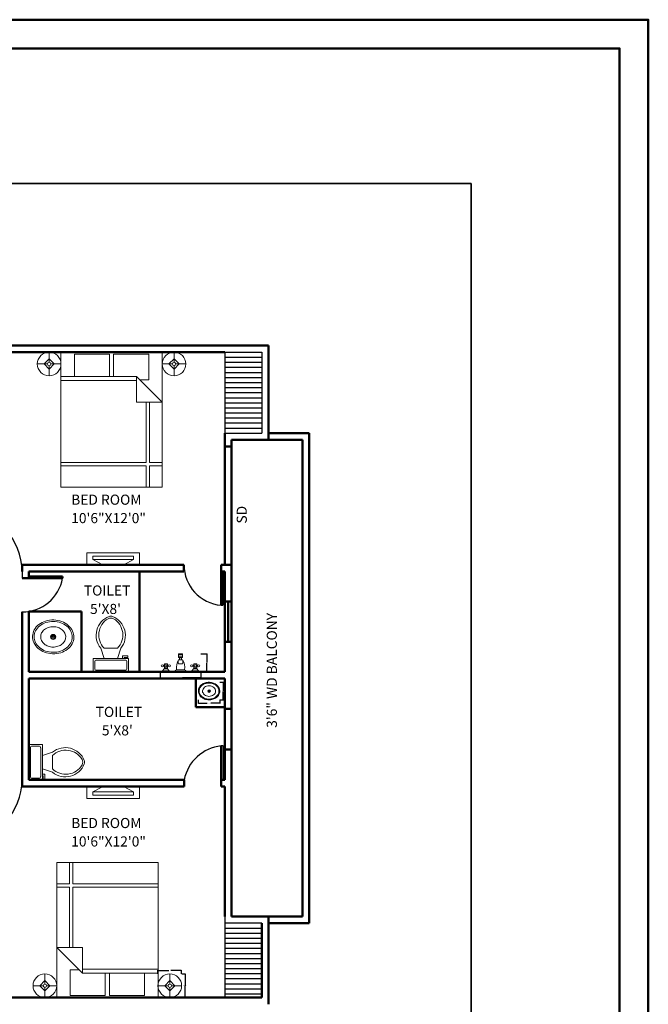
# Model space of a CAD drawing. Units: inches. Extents: x 1493 to 2377, y 814 to 2191.
# Tile 4 of 4: x 2004 to 2377, y 1607 to 2191. Entities that reach past the tile are written whole.
import ezdxf

# ---------------------------------------------------------------- set-up
doc = ezdxf.new("R2010")
doc.units = ezdxf.units.IN
for name, color, linetype, lineweight in [('A-ANNO-DIMS', 2, 'Continuous', 18), ('A-ANNO-TTLB', 7, 'Continuous', 35), ('A-AREA-IDEN', 7, 'Continuous', 18), ('A-DOOR', 4, 'Continuous', 25), ('A-EQPM', 9, 'Continuous', 18), ('A-FLOR-FIXT', 8, 'Continuous', 18), ('A-FURN', 8, 'Continuous', 18), ('A-GLAZ', 4, 'Continuous', 25), ('A-WALL', 7, 'Continuous', 50)]:
    doc.layers.add(name, color=color, linetype=linetype, lineweight=lineweight)
doc.styles.get("Standard").update_dxf_attribs({"font": 'arial.ttf'})
doc.dimstyles.get("Standard").update_dxf_attribs({"dimtxt": 0.18, "dimasz": 0.18, "dimexe": 0.18, "dimexo": 0.0625, "dimgap": 0.09, "dimtad": 0, "dimtih": 1, "dimtoh": 1, "dimdec": 4, "dimzin": 0, "dimdsep": 46, "dimtxsty": 'Standard', "dimcen": 0.09, "dimadec": 0, "dimazin": 0, "dimtfac": 1, "dimtdec": 4, "dimtofl": 0, "dimtmove": 0, "dimatfit": 3, "dimfxl": 1, "dimtolj": 1, "dimtzin": 0, "dimarcsym": 0})

# ---------------------------------------------------------------- blocks, each defined once
blk = doc.blocks.new('Lamp - Table')
for p, q in [((0, 7), (0, 1)), ((-1, 0), (-7, 0)), ((0, 3), (-3, 0)), ((-3, 0), (0, -3)), ((3, 0), (0, 3)), ((0, -3), (3, 0)), ((1, 0), (7, 0)), ((0, -1), (0, -7))]:
    blk.add_line(p, q)
for radius in [7, 1]:
    blk.add_circle((0, 0), radius)
blk = doc.blocks.new('Bed - Queen')
for p, q in [((0, -80), (0, 0)), ((0, 0), (60, 0)), ((60, 0), (60, -80)), ((8, -1.2), (28.8, -1.2)), ((8, -14.4), (8, -1.2)), ((28.8, -1.2), (28.8, -14.4)), ((31.2, -1.2), (52, -1.2)), ((31.2, -14.4), (31.2, -1.2)), ((52, -1.2), (52, -16.4)), ((0, -14.4), (44.8, -14.4)), ((44.8, -16.8), (0, -16.8)), ((60, -29.6), (44.8, -14.4)), ((44.8, -14.4), (44.8, -29.6)), ((52, -16.4), (46.8, -16.4)), ((44.8, -29.6), (60, -29.6)), ((50.4, -29.6), (50.4, -65.35)), ((52.4, -29.6), (52.4, -65.35)), ((50.4, -65.35), (0, -65.35)), ((50.4, -67.35), (0, -67.35)), ((50.4, -67.35), (50.4, -80)), ((60, -65.35), (52.4, -65.35)), ((60, -67.35), (52.4, -67.35)), ((52.4, -67.35), (52.4, -80)), ((60, -80), (0, -80))]:
    blk.add_line(p, q)
blk = doc.blocks.new('Sink - Oval top')
for p, q in [((-1, 0), (1, 0)), ((0, 1), (0, -1))]:
    blk.add_line(p, q)
for points in [[(-12.23, 0.39, 0.117634), (-11.46, -3.36, 0.104469), (-8.88, -6.8, 0.090016), (-5.08, -9.07, 0.08192), (-0.32, -10.02, 0.08192), (4.49, -9.38, 0.090016), (8.42, -7.36, 0.104469), (11.22, -4.09, 0.117634), (12.23, -0.39, 0.117634), (11.46, 3.36, 0.104469), (8.88, 6.8, 0.090016), (5.08, 9.07, 0.08192), (0.32, 10.02, 0.08192), (-4.49, 9.38, 0.090016), (-8.42, 7.36, 0.104469), (-11.22, 4.09, 0.117634)], [(-11.29, 0.16, 0.118622), (-10.52, -3.25, 0.104678), (-8.07, -6.36, 0.089562), (-4.54, -8.37, 0.081185), (-0.13, -9.15, 0.081185), (4.3, -8.49, 0.089562), (7.89, -6.58, 0.104678), (10.42, -3.55, 0.118622), (11.29, -0.16, 0.118622), (10.52, 3.25, 0.104678), (8.07, 6.36, 0.089562), (4.54, 8.37, 0.081185), (0.13, 9.15, 0.081185), (-4.3, 8.49, 0.089562), (-7.89, 6.58, 0.104678), (-10.42, 3.55, 0.118622)], [(-7.42, 0.08, 0.118283), (-6.91, -2.17, 0.104607), (-5.29, -4.21, 0.089718), (-2.97, -5.53, 0.081436), (-0.07, -6.04, 0.081436), (2.84, -5.59, 0.089718), (5.2, -4.33, 0.104607), (6.86, -2.32, 0.118283), (7.42, -0.08, 0.118283), (6.91, 2.17, 0.104607), (5.29, 4.21, 0.089718), (2.97, 5.53, 0.081436), (0.07, 6.04, 0.081436), (-2.84, 5.59, 0.089718), (-5.2, 4.33, 0.104607), (-6.86, 2.32, 0.118283)]]:
    blk.add_lwpolyline(points, format="xyb", close=True)
for radius in [1.5, 1]:
    blk.add_circle((0, 0), radius)
blk = doc.blocks.new('Toilet - top')
for p, q in [((9.5, -6), (9.5, -2)), ((-10, -8.5), (-8, -8.5)), ((-10, -9.5), (-10, -8.5)), ((-7, -9.5), (-10, -9.5)), ((-8, -8.5), (-8, -8)), ((-7, -8), (-7, -9.5)), ((-4, -8), (-6, -14)), ((4, -8), (6, -14)), ((4, -14), (-4, -14))]:
    blk.add_line(p, q)
blk.add_lwpolyline([(10.5, -8), (10.5, 0), (-10.5, 0), (-10.5, -8)], close=True)
for points in [[(-9.5, -2), (-9.5, -6)], [(8.5, -1), (-8.5, -1)], [(-8.5, -7), (8.5, -7)]]:
    blk.add_lwpolyline(points)
for centre, radius, start, end in [((-8.62, -1.88), 0.884, 81.8699, 188.1301), ((8.62, -1.88), 0.884, 351.8699, 98.1301), ((-8.62, -6.12), 0.884, 171.8699, 278.1301), ((8.62, -6.12), 0.884, 261.8699, 8.1301), ((3.52, -21.58), 12.17, 141.46911, 247.97143), ((4.2, -21.82), 11.33, 136.36773, 238.94682), ((-3.52, -21.58), 12.17, 292.02843, 38.53071), ((-4.2, -21.82), 11.33, 301.05301, 43.63209), ((0, -27.88), 4, 245.73182, 294.26817), ((0, -29), 4, 254.86053, 285.13947)]:
    blk.add_arc(centre, radius, start, end)
blk = doc.blocks.new('Faucet - Bathroom front')
for p, q in [((-0.5, 4.25), (0.5, 4.25)), ((0.5, 3.75), (-0.5, 3.75)), ((-0.5, 3), (0.5, 3)), ((-0.25, 3), (-0.25, 3.5)), ((0.25, 3.5), (0.25, 3)), ((-5, 0), (-2.25, 0)), ((-4.5087, 0.25), (-2.7408, 0.25)), ((-4, 1.625), (-4.25, 1.625)), ((-4, 1.375), (-4.25, 1.375)), ((-3.1442, 0.75), (-4.0979, 0.75)), ((-3.25, 1.625), (-3, 1.625)), ((-3.25, 1.375), (-3, 1.375)), ((-1.5, 0), (1.5, 0)), ((-1, 0.5), (1, 0.5)), ((0.5, 2), (-0.5, 2)), ((2.25, 0), (5, 0)), ((2.7413, 0.25), (4.5092, 0.25)), ((3.25, 1.625), (3, 1.625)), ((3.25, 1.375), (3, 1.375)), ((4.1058, 0.75), (3.1521, 0.75)), ((4, 1.625), (4.25, 1.625)), ((4, 1.375), (4.25, 1.375))]:
    blk.add_line(p, q)
for points in [[(-0.5, 3.75), (-0.5, 4.25)], [(-0.25, 4.5), (0.25, 4.5)], [(0.25, 3.5), (-0.25, 3.5)], [(0.5, 4.25), (0.5, 3.75)]]:
    blk.add_lwpolyline(points)
for points in [[(-4, 1), (-4, 2), (-3.25, 2), (-3.25, 1)], [(3.25, 1), (3.25, 2), (4, 2), (4, 1)]]:
    blk.add_lwpolyline(points, close=True)
for centre in [(-4.5, 1.5), (-3.625, 1.5), (-2.75, 1.5), (2.75, 1.5), (3.625, 1.5), (4.5, 1.5)]:
    blk.add_circle(centre, 0.2795)
for centre, radius, start, end in [((3, 1), 4.0311, 150.2551, 187.125), ((0.6413, 2.5), 1.246, 156.3417, 203.6583), ((-0.2575, 4.2575), 0.2426, 88.22243, 181.7776), ((-0.2575, 3.7425), 0.2426, 178.2224, 271.7776), ((0.2575, 4.2575), 0.2426, 358.2224, 91.77757), ((0.2575, 3.7425), 0.2426, 268.2224, 1.777565), ((-3, 1), 4.0311, 352.875, 29.74488), ((-0.6413, 2.5), 1.246, 336.3417, 23.65835), ((-5.375, 1.375), 1.4252, 285.2551, 344.7449), ((-1.875, 1.375), 1.4252, 195.2551, 254.7449), ((-0.7962, -0.2038), 0.7327, 106.1502, 163.8498), ((0.7962, -0.2038), 0.7327, 16.1502, 73.84979), ((1.875, 1.375), 1.4252, 285.2551, 344.7449), ((5.375, 1.375), 1.4252, 195.2551, 254.7449)]:
    blk.add_arc(centre, radius, start, end)
blk = doc.blocks.new('AC-SPLIT-UNIT')
for p, q in [((-2, 27.5), (-2, -3.65)), ((-2, 27.5), (5, 27.5)), ((0, 24), (2, 24)), ((0, 24), (0, 0)), ((2, 24), (2, 0)), ((2, 24), (5, 18.22)), ((2, 0), (5, 5.78)), ((-2, -3.65), (5, -3.65)), ((0, 0), (2, 0))]:
    blk.add_line(p, q)
blk = doc.blocks.new('*D14')
at = {"layer": 'A-ANNO-DIMS', "color": 0, "lineweight": -2, "transparency": 16777216}
for p, q in [((2100.38, 1625.4), (2102.6, 1625.4)), ((2102.42, 1625.22), (2102.42, 1618.58)), ((2102.42, 1611.58), (2102.42, 1618.22)), ((2100.38, 1611.4), (2102.6, 1611.4))]:
    blk.add_line(p, q, dxfattribs=at)
at = {"layer": 'A-ANNO-DIMS', "color": 0, "transparency": 16777216}
for points in [[(2102.39, 1625.22), (2102.45, 1625.22), (2102.42, 1625.4)], [(2102.39, 1611.58), (2102.45, 1611.58), (2102.42, 1611.4)]]:
    blk.add_solid(points, dxfattribs=at)
at = {"layer": 'Defpoints', "color": 0, "transparency": 16777216}
for p in [(2100.32, 1625.4), (2102.42, 1625.4), (2100.32, 1611.4)]:
    blk.add_point(p, dxfattribs=at)
at = {"layer": 'A-ANNO-DIMS', "color": 0, "transparency": 16777216, "insert": (2102.42, 1618.4), "char_height": 0.18, "attachment_point": 5}
blk.add_mtext('\\A1;BEDSIDE TABLE 14 TYP.', dxfattribs=at)
blk = doc.blocks.new('*D15')
at = {"layer": 'A-ANNO-DIMS', "color": 0, "lineweight": -2, "transparency": 16777216}
for p, q in [((2086.32, 1625.46), (2086.32, 1627.68)), ((2086.5, 1627.5), (2092.8, 1627.5)), ((2100.14, 1627.5), (2093.84, 1627.5)), ((2100.32, 1625.46), (2100.32, 1627.68))]:
    blk.add_line(p, q, dxfattribs=at)
at = {"layer": 'A-ANNO-DIMS', "color": 0, "transparency": 16777216}
for points in [[(2086.5, 1627.53), (2086.5, 1627.47), (2086.32, 1627.5)], [(2100.14, 1627.53), (2100.14, 1627.47), (2100.32, 1627.5)]]:
    blk.add_solid(points, dxfattribs=at)
at = {"layer": 'Defpoints', "color": 0, "transparency": 16777216}
for p in [(2086.32, 1627.5), (2086.32, 1625.4), (2100.32, 1625.4)]:
    blk.add_point(p, dxfattribs=at)
at = {"layer": 'A-ANNO-DIMS', "color": 0, "transparency": 16777216, "insert": (2093.32, 1627.5), "char_height": 0.18, "attachment_point": 5}
blk.add_mtext('\\A1;14 TYP.', dxfattribs=at)
blk = doc.blocks.new('*D18')
at = {"layer": 'A-ANNO-DIMS', "color": 0, "lineweight": -2, "transparency": 16777216}
for p, q in [((2110.19, 1787.71), (2110.19, 1785.68)), ((2110.37, 1785.86), (2115.52, 1785.86)), ((2122.76, 1785.86), (2117.61, 1785.86)), ((2122.94, 1787.71), (2122.94, 1785.68))]:
    blk.add_line(p, q, dxfattribs=at)
at = {"layer": 'A-ANNO-DIMS', "color": 0, "transparency": 16777216}
for points in [[(2110.37, 1785.89), (2110.37, 1785.83), (2110.19, 1785.86)], [(2122.76, 1785.89), (2122.76, 1785.83), (2122.94, 1785.86)]]:
    blk.add_solid(points, dxfattribs=at)
at = {"layer": 'Defpoints', "color": 0, "transparency": 16777216}
for p in [(2110.19, 1787.78), (2122.94, 1787.78), (2122.94, 1785.86)]:
    blk.add_point(p, dxfattribs=at)
at = {"layer": 'A-ANNO-DIMS', "color": 0, "transparency": 16777216, "insert": (2116.57, 1785.86), "char_height": 0.18, "attachment_point": 5}
blk.add_mtext('\\A1;WASH BASIN 13', dxfattribs=at)
blk = doc.blocks.new('*D19')
at = {"layer": 'A-ANNO-DIMS', "color": 0, "lineweight": -2, "transparency": 16777216}
for p, q in [((2123.01, 1798.23), (2125.04, 1798.23)), ((2124.86, 1798.05), (2124.86, 1793.19)), ((2124.86, 1787.96), (2124.86, 1792.82)), ((2123.01, 1787.78), (2125.04, 1787.78))]:
    blk.add_line(p, q, dxfattribs=at)
at = {"layer": 'A-ANNO-DIMS', "color": 0, "transparency": 16777216}
for points in [[(2124.83, 1798.05), (2124.89, 1798.05), (2124.86, 1798.23)], [(2124.83, 1787.96), (2124.89, 1787.96), (2124.86, 1787.78)]]:
    blk.add_solid(points, dxfattribs=at)
at = {"layer": 'Defpoints', "color": 0, "transparency": 16777216}
for p in [(2122.94, 1798.23), (2124.86, 1798.23), (2122.94, 1787.78)]:
    blk.add_point(p, dxfattribs=at)
at = {"layer": 'A-ANNO-DIMS', "color": 0, "transparency": 16777216, "insert": (2124.86, 1793), "char_height": 0.18, "attachment_point": 5}
blk.add_mtext('\\A1;10', dxfattribs=at)
blk = doc.blocks.new('*D38')
at = {"layer": 'A-ANNO-DIMS', "color": 0, "lineweight": -2, "transparency": 16777216}
for p, q in [((2087.69, 1804.3), (2087.69, 1800.59)), ((2111.67, 1804.3), (2111.67, 1800.59)), ((2087.87, 1800.77), (2098.62, 1800.77)), ((2111.49, 1800.77), (2100.74, 1800.77))]:
    blk.add_line(p, q, dxfattribs=at)
at = {"layer": 'A-ANNO-DIMS', "color": 0, "transparency": 16777216}
for points in [[(2087.87, 1800.8), (2087.87, 1800.74), (2087.69, 1800.77)], [(2111.49, 1800.8), (2111.49, 1800.74), (2111.67, 1800.77)]]:
    blk.add_solid(points, dxfattribs=at)
at = {"layer": 'Defpoints', "color": 0, "transparency": 16777216}
for p in [(2087.69, 1804.37), (2111.67, 1804.37), (2111.67, 1800.77)]:
    blk.add_point(p, dxfattribs=at)
at = {"layer": 'A-ANNO-DIMS', "color": 0, "transparency": 16777216, "insert": (2099.68, 1800.77), "char_height": 0.18, "attachment_point": 5}
blk.add_mtext('\\A1;FAUCET 24 TYP.', dxfattribs=at)
blk = doc.blocks.new('*D39')
at = {"layer": 'A-ANNO-DIMS', "color": 0, "lineweight": -2, "transparency": 16777216}
for p, q in [((2111.73, 1815.16), (2115.45, 1815.16)), ((2115.27, 1814.98), (2115.27, 1809.95)), ((2115.27, 1804.55), (2115.27, 1809.58)), ((2111.73, 1804.37), (2115.45, 1804.37))]:
    blk.add_line(p, q, dxfattribs=at)
at = {"layer": 'A-ANNO-DIMS', "color": 0, "transparency": 16777216}
for points in [[(2115.24, 1814.98), (2115.3, 1814.98), (2115.27, 1815.16)], [(2115.24, 1804.55), (2115.3, 1804.55), (2115.27, 1804.37)]]:
    blk.add_solid(points, dxfattribs=at)
at = {"layer": 'Defpoints', "color": 0, "transparency": 16777216}
for p in [(2111.67, 1815.16), (2115.27, 1815.16), (2111.67, 1804.37)]:
    blk.add_point(p, dxfattribs=at)
at = {"layer": 'A-ANNO-DIMS', "color": 0, "transparency": 16777216, "insert": (2115.27, 1809.77), "char_height": 0.18, "attachment_point": 5}
blk.add_mtext('\\A1;11 TYP.', dxfattribs=at)

msp = doc.modelspace()

# ---------------------------------------------------------------- linework, layer by layer
at = {"layer": 'A-ANNO-TTLB'}
for p, q in [((1603.83, 2093.87), (2271.83, 2093.87)), ((2271.83, 2093.87), (2271.83, 914.87))]:
    msp.add_line(p, q, dxfattribs=at)
at = {"layer": 'A-DOOR'}
for p, q in [((2005.83, 1863.87), (2005.85, 1863.87)), ((2005.85, 1863.87), (2005.85, 1859.87)), ((2124.7, 1863.87), (2124.7, 1843.87)), ((2123.7, 1843.87), (2124.7, 1843.87)), ((2124.83, 1760.47), (2123.83, 1760.47)), ((2124.83, 1760.47), (2124.83, 1740.47))]:
    msp.add_line(p, q, dxfattribs=at)
for centre, radius, start, end in [((1969.77, 1863.87), 36.06, 0, 86.72685), ((2125.79, 1867.87), 24.09, 180, 265.02089), ((2005.85, 1864.27), 24.4, 269.96306, 349.61114), ((2126.33, 1735.65), 24.94, 95.73959, 169.10486), ((1969.77, 1740.37), 36.06, 273.27315, 360)]:
    msp.add_arc(centre, radius, start, end, dxfattribs=at)
at = {"layer": 'A-GLAZ'}
for p, q in [((2125.83, 1993.87), (2125.83, 1948.87)), ((2125.83, 1993.87), (2147.83, 1993.87)), ((2125.83, 1990.87), (2147.83, 1990.87)), ((2147.83, 1993.87), (2147.83, 1945.87)), ((2125.83, 1987.87), (2147.83, 1987.87)), ((2125.83, 1984.87), (2147.83, 1984.87)), ((2125.83, 1981.87), (2147.83, 1981.87)), ((2125.83, 1978.87), (2147.83, 1978.87)), ((2125.83, 1975.87), (2147.83, 1975.87)), ((2125.83, 1972.87), (2147.83, 1972.87)), ((2125.83, 1969.87), (2147.83, 1969.87)), ((2125.83, 1966.87), (2147.83, 1966.87)), ((2125.83, 1963.87), (2147.83, 1963.87)), ((2125.83, 1960.87), (2147.83, 1960.87)), ((2125.83, 1957.87), (2147.83, 1957.87)), ((2125.83, 1954.87), (2147.83, 1954.87)), ((2125.83, 1951.87), (2147.83, 1951.87)), ((2125.83, 1948.87), (2147.83, 1948.87)), ((2125.83, 1948.87), (2125.83, 1945.87)), ((2125.83, 1945.87), (2147.83, 1945.87)), ((2125.83, 1659.37), (2125.83, 1611.37)), ((2147.83, 1655.37), (2125.83, 1655.37)), ((2147.83, 1652.37), (2125.83, 1652.37)), ((2147.83, 1649.37), (2125.83, 1649.37)), ((2147.83, 1646.37), (2125.83, 1646.37)), ((2147.83, 1643.37), (2125.83, 1643.37)), ((2147.83, 1640.37), (2125.83, 1640.37)), ((2147.83, 1637.37), (2125.83, 1637.37)), ((2147.83, 1634.37), (2125.83, 1634.37)), ((2147.83, 1631.37), (2125.83, 1631.37)), ((2147.83, 1628.37), (2125.83, 1628.37)), ((2147.83, 1625.37), (2125.83, 1625.37)), ((2147.83, 1622.37), (2125.83, 1622.37)), ((2147.83, 1619.37), (2125.83, 1619.37)), ((2147.83, 1616.37), (2125.83, 1616.37)), ((2147.83, 1613.37), (2125.83, 1613.37))]:
    msp.add_line(p, q, dxfattribs=at)
at = {"layer": 'A-WALL'}
for p, q in [((1965.83, 1997.87), (2151.83, 1997.87)), ((2007.83, 1997.87), (2011.83, 1997.87)), ((2151.83, 1997.87), (2151.83, 1941.87)), ((1969.83, 1993.87), (2125.83, 1993.87)), ((2125.83, 1945.87), (2125.83, 1867.87)), ((2151.83, 1945.87), (2175.83, 1945.87)), ((2175.83, 1945.87), (2175.83, 1655.37)), ((2125.83, 1937.87), (2129.83, 1937.87)), ((2129.83, 1941.87), (2171.83, 1941.87)), ((2129.83, 1941.87), (2129.83, 1659.37)), ((2171.83, 1941.87), (2171.83, 1659.37)), ((2005.83, 1867.87), (2005.83, 1863.87)), ((2005.83, 1867.87), (2101.7, 1867.87)), ((2005.83, 1867.87), (2005.83, 1863.87)), ((2101.7, 1867.87), (2101.7, 1863.87)), ((2123.7, 1867.87), (2123.7, 1843.87)), ((2123.7, 1867.87), (2129.83, 1867.87)), ((2009.83, 1863.87), (2009.83, 1859.87)), ((2009.83, 1863.87), (2101.7, 1863.87)), ((2075.31, 1863.87), (2075.31, 1804.37)), ((2123.7, 1863.87), (2125.83, 1863.87)), ((2125.83, 1863.87), (2125.83, 1804.37)), ((2005.85, 1859.87), (2029.85, 1859.87)), ((2009.85, 1860.87), (2029.85, 1860.87)), ((2029.85, 1860.87), (2029.85, 1859.87)), ((2125.83, 1846.12), (2129.83, 1846.12)), ((2127.83, 1846.12), (2127.83, 1822.12)), ((2005.83, 1839.87), (2005.83, 1736.37)), ((2009.83, 1840.19), (2009.83, 1804.37)), ((2009.83, 1840.19), (2040.96, 1840.19)), ((2040.96, 1840.19), (2040.96, 1804.37)), ((2125.83, 1822.12), (2129.83, 1822.12)), ((2125.83, 1804.37), (2009.83, 1804.37)), ((2125.83, 1800.37), (2009.83, 1800.37)), ((2009.83, 1800.37), (2009.83, 1740.37)), ((2108.83, 1800.37), (2108.83, 1783.37)), ((2125.83, 1800.37), (2125.83, 1740.47)), ((2125.83, 1783.37), (2108.83, 1783.37)), ((2125.83, 1782.42), (2129.83, 1782.42)), ((2123.83, 1760.47), (2123.83, 1736.47)), ((2125.83, 1758.42), (2129.83, 1758.42)), ((2101.83, 1740.37), (2009.83, 1740.37)), ((2101.83, 1740.47), (2101.83, 1736.37)), ((2125.83, 1740.47), (2123.83, 1740.47)), ((2101.83, 1736.37), (2005.83, 1736.37)), ((2125.83, 1736.47), (2123.83, 1736.47)), ((2125.83, 1736.47), (2125.83, 1659.37)), ((2171.83, 1659.37), (2129.83, 1659.37)), ((2151.83, 1659.37), (2151.83, 1607.37)), ((2147.83, 1655.37), (2147.83, 1611.37)), ((2175.83, 1655.37), (2151.83, 1655.37)), ((2147.83, 1611.37), (1964.83, 1611.37))]:
    msp.add_line(p, q, dxfattribs=at)
for points in [[(1493.21, 2190.87), (2376.73, 2190.87), (2376.73, 813.94), (1493.21, 813.94)], [(1510.21, 2173.87), (2359.73, 2173.87), (2359.73, 830.94), (1510.21, 830.94)]]:
    msp.add_lwpolyline(points, close=True, dxfattribs=at)

# ---------------------------------------------------------------- block references
at = {"layer": 'A-EQPM'}
for p, rotation in [((2047.81, 1872.87), 270.0000000000077), ((2071.76, 1731.37), 90.08441836094227)]:
    msp.add_blockref('AC-SPLIT-UNIT', p, dxfattribs=dict(at, rotation=rotation))
at = {"layer": 'A-FLOR-FIXT'}
msp.add_blockref('Sink - Oval top', (2024.25, 1825.11), dxfattribs=at)
for p, rotation in [((2058.37, 1804.37), 179.999999999999), ((2009.83, 1750.84), 89.99999999999905)]:
    msp.add_blockref('Toilet - top', p, dxfattribs=dict(at, rotation=rotation))
for name, p, xscale, yscale, zscale in [('Faucet - Bathroom front', (2099.68, 1804.37), 2.398174673042902, 2.398174673042902, 2.398174673042902), ('Sink - Oval top', (2116.57, 1793), 0.5193570426410568, 0.5193570426410568, 0.5193570426410568)]:
    msp.add_blockref(name, p, dxfattribs=dict(at, xscale=xscale, yscale=yscale, zscale=zscale))
at = {"layer": 'A-FURN'}
for name, p, rotation in [('Lamp - Table', (2021.85, 1986.83), 270), ('Lamp - Table', (2095.83, 1986.83), 270), ('Bed - Queen', (2086.33, 1611.37), 180), ('Lamp - Table', (2019.33, 1618.4), 89.99999999999999), ('Lamp - Table', (2093.32, 1618.4), 89.99999999999999)]:
    msp.add_blockref(name, p, dxfattribs=dict(at, rotation=rotation))
msp.add_blockref('Bed - Queen', (2028.83, 1993.87), dxfattribs=at)

# ---------------------------------------------------------------- texts
at = {"layer": 'A-AREA-IDEN'}
for s, p in [('BED ROOM', (2034.91, 1903.42)), ('10\'6"X12\'0"', (2034.91, 1892.5)), ('TOILET', (2042.4, 1849.59)), ("  5'X8'", (2042.4, 1838.67)), ('TOILET', (2049.41, 1777.66)), ("  5'X8'", (2049.41, 1766.73)), ('BED ROOM', (2034.91, 1711.8)), ('10\'6"X12\'0"', (2034.91, 1700.88))]:
    msp.add_text(s, height=6, dxfattribs=at).set_placement(p)
for s, p in [('      SD', (2138.93, 1881.25)), ('3\'6" WD BALCONY', (2156.75, 1771.22))]:
    msp.add_text(s, height=6, rotation=90, dxfattribs=at).set_placement(p)

# ---------------------------------------------------------------- dimensions: what is measured, and where the dimension line sits
at = {"layer": 'A-ANNO-DIMS'}
for base, p1, p2, angle, text, picture, middle in [((2115.27, 1815.16), (2111.67, 1804.37), (2111.67, 1815.16), 90, '<> TYP.', '*D39', (2115.27, 1809.77)), ((2086.32, 1627.5), (2100.32, 1625.4), (2086.32, 1625.4), 180, '<> TYP.', '*D15', (2093.32, 1627.5)), ((2102.42, 1625.4), (2100.32, 1611.4), (2100.32, 1625.4), 90, 'BEDSIDE TABLE <> TYP.', '*D14', (2102.42, 1618.4))]:
    dim = msp.add_linear_dim(base=base, p1=p1, p2=p2, angle=angle, text=text, dimstyle='Standard', override={"dimdec": 0, "dimlfac": 1, "dimrnd": 0, "dimzin": 0, "dimdsep": 46, "dimlunit": 2}, dxfattribs=at)
    dim.commit()
    dim.dimension.update_dxf_attribs({"geometry": picture, "text_midpoint": middle})
for base, p1, p2, text, picture, middle in [((2111.67, 1800.77), (2087.69, 1804.37), (2111.67, 1804.37), 'FAUCET <> TYP.', '*D38', (2099.68, 1800.77)), ((2122.94, 1785.86), (2110.19, 1787.78), (2122.94, 1787.78), 'WASH BASIN <>', '*D18', (2116.57, 1785.86))]:
    dim = msp.add_linear_dim(base=base, p1=p1, p2=p2, text=text, dimstyle='Standard', override={"dimdec": 0, "dimlfac": 1, "dimrnd": 0, "dimzin": 0, "dimdsep": 46, "dimlunit": 2}, dxfattribs=at)
    dim.commit()
    dim.dimension.update_dxf_attribs({"geometry": picture, "text_midpoint": middle})
dim = msp.add_linear_dim(base=(2124.86, 1798.23), p1=(2122.94, 1787.78), p2=(2122.94, 1798.23), angle=90, dimstyle='Standard', override={"dimdec": 0, "dimlfac": 1, "dimrnd": 0, "dimzin": 0, "dimdsep": 46, "dimlunit": 2}, dxfattribs=at)
dim.commit()
dim.dimension.update_dxf_attribs({"geometry": '*D19', "text_midpoint": (2124.86, 1793)})

doc.saveas('drawing.dxf')
